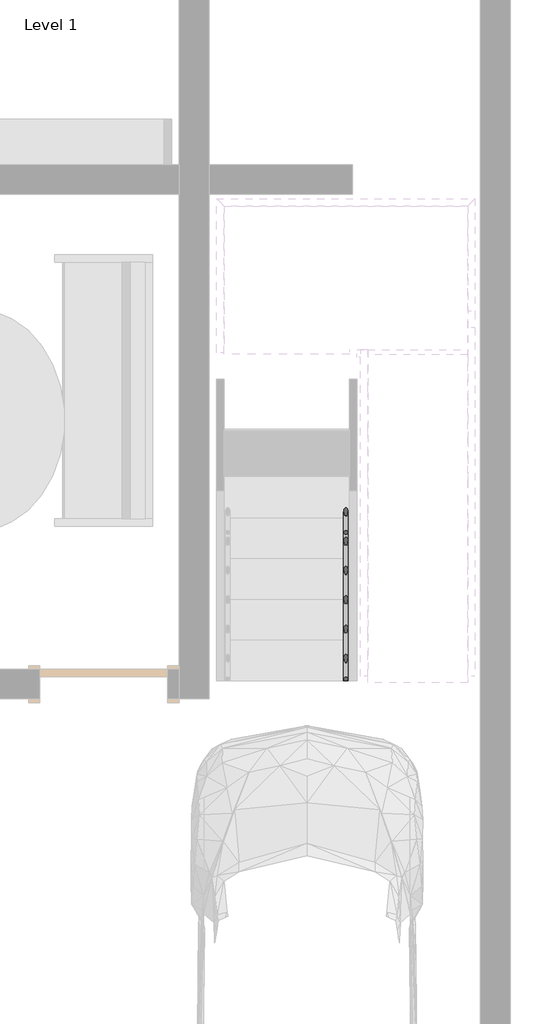
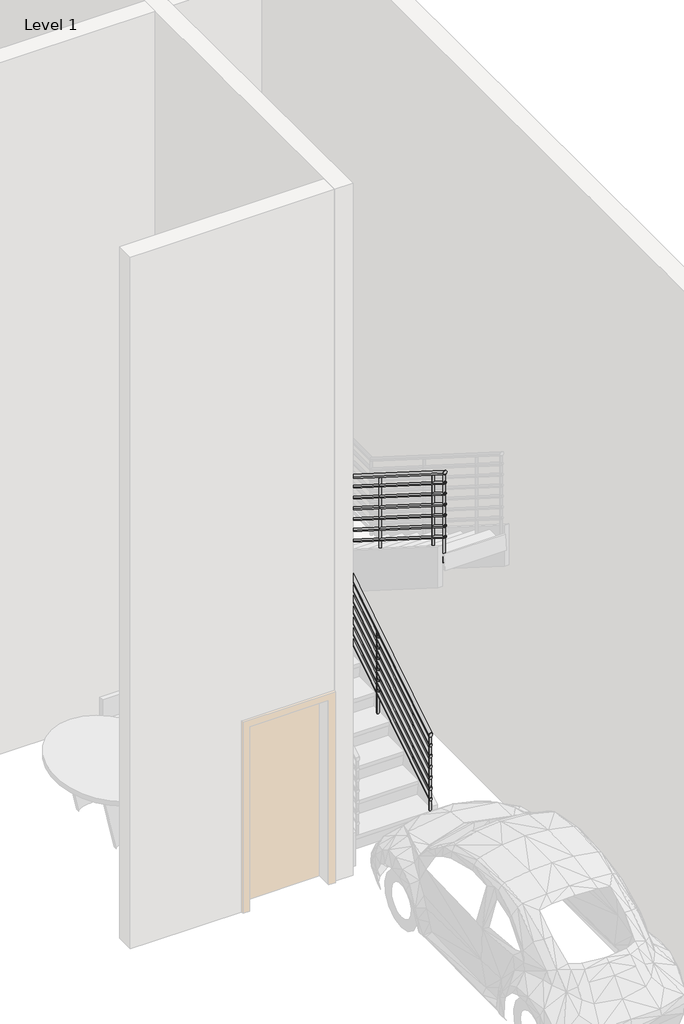
# One storey, part 2 of 4: 1 railing.
"""IFC4 building model written with IfcOpenShell, lengths in millimetres."""

from ifc_helpers import new_model, si_unit, point, frame, frame_2d, origin, place, context, project, spatial, circle_curve, ellipse_curve, trimmed, segment, composite_curve, outline, extrude, element, save
from ifc_brep_helpers import plane_surface, cylinder_surface, advanced_brep

model = new_model("IFC4")

# Units and contexts
model_context = context("Model", 3, world=origin())
ifc_project = project(units=[si_unit("LENGTHUNIT", "METRE", prefix="MILLI")], contexts=[model_context])

# Site, building, storey
site = spatial("IfcSite", under=ifc_project)
building = spatial("IfcBuilding", under=site)
storey = spatial("IfcBuildingStorey", under=building, Name="Level 1", Elevation=0.0)

# Railing
placement = place(None, origin())
element("IfcRailing", 1, ObjectType="900mm Pipe", at=placement, inside=storey, context=model_context, shape_type="SolidModel", body=[
    advanced_brep(
    [(474.1868738, 5121.4805518, 1224.1622432), (434.1868738, 5121.4805518, 1224.1622432), (474.1868738, 7327.2740048, 2619.1304348), (434.1868738, 7327.2740048, 2619.1304348), (474.1868738, 7356.6805518, 2619.1304348), (434.1868738, 7396.6805518, 2619.1304348), (627.5868738, 7356.6805518, 2619.1304348), (627.5868738, 7396.6805518, 2619.1304348)],
    [
        (0, 1, ellipse_curve(frame((454.1868738, 5121.4805518, 1224.1622432), z_axis=(0.0, -1.0, 0.0), x_axis=(0.0, 0.0, -1.0)), 23.6638438, 20.0)),
        (1, 0, ellipse_curve(frame((454.1868738, 5121.4805518, 1224.1622432), z_axis=(0.0, -1.0, 0.0), x_axis=(0.0, 0.0, -1.0)), 23.6638438, 20.0)),
        (0, 2),
        (2, 3, ellipse_curve(frame((454.1868738, 7327.2740048, 2619.1304348), z_axis=(0.0, -0.9605132043335073, -0.2782344053149755), x_axis=(0.0, 0.27823440531497556, -0.9605132043335073)), 20.822202, 20.0)),
        (3, 1),
        (3, 2, ellipse_curve(frame((454.1868738, 7327.2740048, 2619.1304348), z_axis=(0.0, -0.9605132043335073, -0.2782344053149755), x_axis=(0.0, 0.27823440531497556, -0.9605132043335073)), 20.822202, 20.0)),
        (2, 4),
        (4, 5, ellipse_curve(frame((454.1868738, 7376.6805518, 2619.1304348), z_axis=(-0.7071067811865482, -0.7071067811865467, 0.0), x_axis=(0.7071067811865466, -0.7071067811865485, 0.0)), 28.2842712, 20.0)),
        (5, 3),
        (5, 4, ellipse_curve(frame((454.1868738, 7376.6805518, 2619.1304348), z_axis=(-0.7071067811865482, -0.7071067811865467, 0.0), x_axis=(0.7071067811865466, -0.7071067811865485, 0.0)), 28.2842712, 20.0)),
        (6, 7, ellipse_curve(frame((627.5868738, 7376.6805518, 2619.1304348), z_axis=(0.7071067811865476, 0.0, 0.7071067811865476), x_axis=(-0.7071067811865474, 0.0, 0.7071067811865478)), 28.2842712, 20.0)),
        (7, 6, ellipse_curve(frame((627.5868738, 7376.6805518, 2619.1304348), z_axis=(0.7071067811865476, 0.0, 0.7071067811865476), x_axis=(-0.7071067811865474, 0.0, 0.7071067811865478)), 28.2842712, 20.0)),
        (4, 6),
        (7, 5),
    ],
    [
        plane_surface(frame((454.1868738, 5121.4805518, 1247.826087), z_axis=(0.0, -1.0, 0.0), x_axis=(0.0, 0.0, 1.0))),
        cylinder_surface(frame((454.1868738, 5132.1704646, 1230.9226623), z_axis=(0.0, -0.8451712313980438, -0.5344956404098301), x_axis=(-1.0, 0.0, 0.0)), 20.0),
        cylinder_surface(frame((454.1868738, 7321.4805518, 2619.1304348), z_axis=(0.0, -1.0, 0.0), x_axis=(-1.0, 0.0, 0.0)), 20.0),
        plane_surface(frame((607.5868738, 7376.6805518, 2639.1304348), z_axis=(0.7071067811865476, 0.0, 0.7071067811865476), x_axis=(0.7071067811865476, 0.0, -0.7071067811865476))),
        cylinder_surface(frame((454.1868738, 7376.6805518, 2619.1304348), z_axis=(-1.0, 0.0, 0.0), x_axis=(0.0, 1.0, 0.0)), 20.0),
    ],
    [
        (0, [[1, 2]]),
        (1, [[-1, 3, 4, 5]]),
        (1, [[-2, -5, 6, -3]]),
        (2, [[-4, 7, 8, 9]]),
        (2, [[-6, -9, 10, -7]]),
        (3, [[11, 12]]),
        (4, [[-8, 13, -12, 14]]),
        (4, [[-10, -14, -11, -13]]),
    ],
),
    advanced_brep(
    [(627.5868738, 7356.6805518, 2619.1304348), (627.5868738, 7396.6805518, 2619.1304348), (627.5868738, 7356.6805518, 2762.3007709), (627.5868738, 7396.6805518, 2784.3320158)],
    [
        (0, 1, ellipse_curve(frame((627.5868738, 7376.6805518, 2619.1304348), z_axis=(-0.7071067811865476, 0.0, -0.7071067811865476), x_axis=(0.7071067811865476, 0.0, -0.7071067811865474)), 28.2842712, 20.0)),
        (1, 0, ellipse_curve(frame((627.5868738, 7376.6805518, 2619.1304348), z_axis=(-0.7071067811865476, 0.0, -0.7071067811865476), x_axis=(0.7071067811865476, 0.0, -0.7071067811865474)), 28.2842712, 20.0)),
        (2, 3, ellipse_curve(frame((627.5868738, 7376.6805518, 2773.3163934), z_axis=(0.0, -0.4824439654458173, 0.8759268349610686), x_axis=(0.0, -0.8759268349610686, -0.48244396544581714)), 22.8329573, 20.0)),
        (3, 2, ellipse_curve(frame((627.5868738, 7376.6805518, 2773.3163934), z_axis=(0.0, -0.4824439654458173, 0.8759268349610686), x_axis=(0.0, -0.8759268349610686, -0.48244396544581714)), 22.8329573, 20.0)),
        (0, 2),
        (3, 1),
    ],
    [
        plane_surface(frame((627.5868738, 7376.6805518, 2619.1304348), z_axis=(-0.7071067811865476, 0.0, -0.7071067811865476), x_axis=(0.7071067811865476, 0.0, -0.7071067811865476))),
        plane_surface(frame((627.5868738, 7376.6805518, 2773.3163934), z_axis=(0.0, -0.4824439654458173, 0.8759268349610686), x_axis=(1.0, 0.0, 0.0))),
        cylinder_surface(frame((627.5868738, 7376.6805518, 2619.1304348), z_axis=(0.0, 0.0, -1.0), x_axis=(0.0, 1.0, 0.0)), 20.0),
    ],
    [
        (0, [[1, 2]]),
        (1, [[3, 4]]),
        (2, [[-1, 5, -4, 6]]),
        (2, [[-2, -6, -3, -5]]),
    ],
),
    advanced_brep(
    [(607.5868738, 7376.6805518, 2773.3163934), (647.5868738, 7376.6805518, 2773.3163934), (607.5868738, 5151.2805518, 4180.6839823), (647.5868738, 5151.2805518, 4180.6839823)],
    [
        (0, 1, ellipse_curve(frame((627.5868738, 7376.6805518, 2773.3163934), z_axis=(0.0, 0.4824439654458173, -0.8759268349610686), x_axis=(0.0, 0.8759268349610685, 0.4824439654458175)), 22.8329573, 20.0)),
        (1, 0, ellipse_curve(frame((627.5868738, 7376.6805518, 2773.3163934), z_axis=(0.0, 0.4824439654458173, -0.8759268349610686), x_axis=(0.0, 0.8759268349610685, 0.4824439654458175)), 22.8329573, 20.0)),
        (2, 3, ellipse_curve(frame((627.5868738, 5151.2805518, 4180.6839823), z_axis=(0.0, -1.0, 0.0), x_axis=(0.0, 0.0, -1.0)), 23.6638438, 20.0)),
        (3, 2, ellipse_curve(frame((627.5868738, 5151.2805518, 4180.6839823), z_axis=(0.0, -1.0, 0.0), x_axis=(0.0, 0.0, -1.0)), 23.6638438, 20.0)),
        (0, 2),
        (3, 1),
    ],
    [
        plane_surface(frame((627.5868738, 7396.6805518, 2784.3320158), z_axis=(0.0, 0.4824439654458173, -0.8759268349610686), x_axis=(1.0, 0.0, 0.0))),
        plane_surface(frame((627.5868738, 5151.2805518, 4204.3478261), z_axis=(0.0, -1.0, 0.0), x_axis=(0.0, 0.0, -1.0))),
        cylinder_surface(frame((627.5868738, 7385.990639, 2767.4285912), z_axis=(0.0, 0.8451712313980438, -0.5344956404098301), x_axis=(1.0, 0.0, 0.0)), 20.0),
    ],
    [
        (0, [[1, 2]]),
        (1, [[3, 4]]),
        (2, [[-1, 5, -4, 6]]),
        (2, [[-2, -6, -3, -5]]),
    ],
),
    advanced_brep(
    [(439.1868738, 5121.4805518, 1105.0782041), (469.1868738, 5121.4805518, 1105.0782041), (439.1868738, 7325.8256416, 2499.1304348), (469.1868738, 7325.8256416, 2499.1304348), (439.1868738, 7391.6805518, 2499.1304348), (469.1868738, 7361.6805518, 2499.1304348), (612.5868738, 7391.6805518, 2499.1304348), (612.5868738, 7361.6805518, 2499.1304348)],
    [
        (0, 1, ellipse_curve(frame((454.1868738, 5121.4805518, 1105.0782041), z_axis=(0.0, -1.0, 0.0), x_axis=(0.0, 0.0, -1.0)), 17.7478828, 15.0)),
        (1, 0, ellipse_curve(frame((454.1868738, 5121.4805518, 1105.0782041), z_axis=(0.0, -1.0, 0.0), x_axis=(0.0, 0.0, -1.0)), 17.7478828, 15.0)),
        (0, 2),
        (2, 3, ellipse_curve(frame((454.1868738, 7325.8256416, 2499.1304348), z_axis=(0.0, -0.9605132043335073, -0.2782344053149755), x_axis=(0.0, 0.27823440531497534, -0.9605132043335074)), 15.6166515, 15.0)),
        (3, 1),
        (3, 2, ellipse_curve(frame((454.1868738, 7325.8256416, 2499.1304348), z_axis=(0.0, -0.9605132043335073, -0.2782344053149755), x_axis=(0.0, 0.27823440531497534, -0.9605132043335074)), 15.6166515, 15.0)),
        (2, 4),
        (4, 5, ellipse_curve(frame((454.1868738, 7376.6805518, 2499.1304348), z_axis=(-0.7071067811865482, -0.7071067811865467, 0.0), x_axis=(0.7071067811865466, -0.7071067811865485, 0.0)), 21.2132034, 15.0)),
        (5, 3),
        (5, 4, ellipse_curve(frame((454.1868738, 7376.6805518, 2499.1304348), z_axis=(-0.7071067811865482, -0.7071067811865467, 0.0), x_axis=(0.7071067811865466, -0.7071067811865485, 0.0)), 21.2132034, 15.0)),
        (6, 7, circle_curve(frame((612.5868738, 7376.6805518, 2499.1304348), z_axis=(1.0, 0.0, 0.0), x_axis=(0.0, -1.0, 0.0)), 15.0)),
        (7, 6, circle_curve(frame((612.5868738, 7376.6805518, 2499.1304348), z_axis=(1.0, 0.0, 0.0), x_axis=(0.0, -1.0, 0.0)), 15.0)),
        (4, 6),
        (7, 5),
    ],
    [
        plane_surface(frame((454.1868738, 5121.4805518, 1122.826087), z_axis=(0.0, -1.0, 0.0), x_axis=(0.0, 0.0, 1.0))),
        cylinder_surface(frame((454.1868738, 5129.4979864, 1110.1485185), z_axis=(0.0, -0.845171231398044, -0.53449564040983), x_axis=(1.0, 0.0, 0.0)), 15.0),
        cylinder_surface(frame((454.1868738, 7321.4805518, 2499.1304348), z_axis=(0.0, -1.0, 0.0), x_axis=(1.0, 0.0, 0.0)), 15.0),
        plane_surface(frame((612.5868738, 7376.6805518, 2514.1304348), z_axis=(1.0, 0.0, 0.0), x_axis=(0.0, 1.0, 0.0))),
        cylinder_surface(frame((454.1868738, 7376.6805518, 2499.1304348), z_axis=(-1.0, 0.0, 0.0), x_axis=(0.0, -1.0, 0.0)), 15.0),
    ],
    [
        (0, [[1, 2]]),
        (1, [[-1, 3, 4, 5]]),
        (1, [[-2, -5, 6, -3]]),
        (2, [[-4, 7, 8, 9]]),
        (2, [[-6, -9, 10, -7]]),
        (3, [[11, 12]]),
        (4, [[-8, 13, -12, 14]]),
        (4, [[-10, -14, -11, -13]]),
    ],
),
    advanced_brep(
    [(642.5868738, 7391.6805518, 2644.7461883), (612.5868738, 7391.6805518, 2644.7461883), (642.5868738, 5151.2805518, 4061.5999432), (612.5868738, 5151.2805518, 4061.5999432)],
    [
        (0, 1, ellipse_curve(frame((627.5868738, 7391.6805518, 2644.7461883), z_axis=(0.0, 1.0, 0.0), x_axis=(0.0, 0.0, -1.0)), 17.7478828, 15.0)),
        (1, 0, ellipse_curve(frame((627.5868738, 7391.6805518, 2644.7461883), z_axis=(0.0, 1.0, 0.0), x_axis=(0.0, 0.0, -1.0)), 17.7478828, 15.0)),
        (2, 3, ellipse_curve(frame((627.5868738, 5151.2805518, 4061.5999432), z_axis=(0.0, -1.0, 0.0), x_axis=(0.0, 0.0, -1.0)), 17.7478828, 15.0)),
        (3, 2, ellipse_curve(frame((627.5868738, 5151.2805518, 4061.5999432), z_axis=(0.0, -1.0, 0.0), x_axis=(0.0, 0.0, -1.0)), 17.7478828, 15.0)),
        (0, 2),
        (3, 1),
    ],
    [
        plane_surface(frame((627.5868738, 7391.6805518, 2662.4940711), z_axis=(0.0, 1.0, 0.0), x_axis=(0.0, 0.0, -1.0))),
        plane_surface(frame((627.5868738, 5151.2805518, 4079.3478261), z_axis=(0.0, -1.0, 0.0), x_axis=(0.0, 0.0, -1.0))),
        cylinder_surface(frame((627.5868738, 7383.6631172, 2649.8165027), z_axis=(0.0, 0.8451712313980437, -0.5344956404098302), x_axis=(-1.0, 0.0, 0.0)), 15.0),
    ],
    [
        (0, [[1, 2]]),
        (1, [[3, 4]]),
        (2, [[-1, 5, -4, 6]]),
        (2, [[-2, -6, -3, -5]]),
    ],
),
    advanced_brep(
    [(439.1868738, 5121.4805518, 980.0782041), (469.1868738, 5121.4805518, 980.0782041), (439.1868738, 7325.8256416, 2374.1304348), (469.1868738, 7325.8256416, 2374.1304348), (439.1868738, 7391.6805518, 2374.1304348), (469.1868738, 7361.6805518, 2374.1304348), (612.5868738, 7391.6805518, 2374.1304348), (612.5868738, 7361.6805518, 2374.1304348)],
    [
        (0, 1, ellipse_curve(frame((454.1868738, 5121.4805518, 980.0782041), z_axis=(0.0, -1.0, 0.0), x_axis=(0.0, 0.0, -1.0)), 17.7478828, 15.0)),
        (1, 0, ellipse_curve(frame((454.1868738, 5121.4805518, 980.0782041), z_axis=(0.0, -1.0, 0.0), x_axis=(0.0, 0.0, -1.0)), 17.7478828, 15.0)),
        (0, 2),
        (2, 3, ellipse_curve(frame((454.1868738, 7325.8256416, 2374.1304348), z_axis=(0.0, -0.9605132043335073, -0.2782344053149755), x_axis=(0.0, 0.27823440531497556, -0.9605132043335073)), 15.6166515, 15.0)),
        (3, 1),
        (3, 2, ellipse_curve(frame((454.1868738, 7325.8256416, 2374.1304348), z_axis=(0.0, -0.9605132043335073, -0.2782344053149755), x_axis=(0.0, 0.27823440531497556, -0.9605132043335073)), 15.6166515, 15.0)),
        (2, 4),
        (4, 5, ellipse_curve(frame((454.1868738, 7376.6805518, 2374.1304348), z_axis=(-0.7071067811865482, -0.7071067811865467, 0.0), x_axis=(0.7071067811865466, -0.7071067811865485, 0.0)), 21.2132034, 15.0)),
        (5, 3),
        (5, 4, ellipse_curve(frame((454.1868738, 7376.6805518, 2374.1304348), z_axis=(-0.7071067811865482, -0.7071067811865467, 0.0), x_axis=(0.7071067811865466, -0.7071067811865485, 0.0)), 21.2132034, 15.0)),
        (6, 7, circle_curve(frame((612.5868738, 7376.6805518, 2374.1304348), z_axis=(1.0, 0.0, 0.0), x_axis=(0.0, -1.0, 0.0)), 15.0)),
        (7, 6, circle_curve(frame((612.5868738, 7376.6805518, 2374.1304348), z_axis=(1.0, 0.0, 0.0), x_axis=(0.0, -1.0, 0.0)), 15.0)),
        (4, 6),
        (7, 5),
    ],
    [
        plane_surface(frame((454.1868738, 5121.4805518, 997.826087), z_axis=(0.0, -1.0, 0.0), x_axis=(0.0, 0.0, 1.0))),
        cylinder_surface(frame((454.1868738, 5129.4979864, 985.1485185), z_axis=(0.0, -0.8451712313980438, -0.5344956404098301), x_axis=(1.0, 0.0, 0.0)), 15.0),
        cylinder_surface(frame((454.1868738, 7321.4805518, 2374.1304348), z_axis=(0.0, -1.0, 0.0), x_axis=(1.0, 0.0, 0.0)), 15.0),
        plane_surface(frame((612.5868738, 7376.6805518, 2389.1304348), z_axis=(1.0, 0.0, 0.0), x_axis=(0.0, 1.0, 0.0))),
        cylinder_surface(frame((454.1868738, 7376.6805518, 2374.1304348), z_axis=(-1.0, 0.0, 0.0), x_axis=(0.0, -1.0, 0.0)), 15.0),
    ],
    [
        (0, [[1, 2]]),
        (1, [[-1, 3, 4, 5]]),
        (1, [[-2, -5, 6, -3]]),
        (2, [[-4, 7, 8, 9]]),
        (2, [[-6, -9, 10, -7]]),
        (3, [[11, 12]]),
        (4, [[-8, 13, -12, 14]]),
        (4, [[-10, -14, -11, -13]]),
    ],
),
    advanced_brep(
    [(642.5868738, 7391.6805518, 2519.7461883), (612.5868738, 7391.6805518, 2519.7461883), (642.5868738, 5151.2805518, 3936.5999432), (612.5868738, 5151.2805518, 3936.5999432)],
    [
        (0, 1, ellipse_curve(frame((627.5868738, 7391.6805518, 2519.7461883), z_axis=(0.0, 1.0, 0.0), x_axis=(0.0, 0.0, -1.0)), 17.7478828, 15.0)),
        (1, 0, ellipse_curve(frame((627.5868738, 7391.6805518, 2519.7461883), z_axis=(0.0, 1.0, 0.0), x_axis=(0.0, 0.0, -1.0)), 17.7478828, 15.0)),
        (2, 3, ellipse_curve(frame((627.5868738, 5151.2805518, 3936.5999432), z_axis=(0.0, -1.0, 0.0), x_axis=(0.0, 0.0, -1.0)), 17.7478828, 15.0)),
        (3, 2, ellipse_curve(frame((627.5868738, 5151.2805518, 3936.5999432), z_axis=(0.0, -1.0, 0.0), x_axis=(0.0, 0.0, -1.0)), 17.7478828, 15.0)),
        (0, 2),
        (3, 1),
    ],
    [
        plane_surface(frame((627.5868738, 7391.6805518, 2537.4940711), z_axis=(0.0, 1.0, 0.0), x_axis=(0.0, 0.0, -1.0))),
        plane_surface(frame((627.5868738, 5151.2805518, 3954.3478261), z_axis=(0.0, -1.0, 0.0), x_axis=(0.0, 0.0, -1.0))),
        cylinder_surface(frame((627.5868738, 7383.6631172, 2524.8165027), z_axis=(0.0, 0.8451712313980438, -0.5344956404098301), x_axis=(-1.0, 0.0, 0.0)), 15.0),
    ],
    [
        (0, [[1, 2]]),
        (1, [[3, 4]]),
        (2, [[-1, 5, -4, 6]]),
        (2, [[-2, -6, -3, -5]]),
    ],
),
    advanced_brep(
    [(439.1868738, 5121.4805518, 855.0782041), (469.1868738, 5121.4805518, 855.0782041), (439.1868738, 7325.8256416, 2249.1304348), (469.1868738, 7325.8256416, 2249.1304348), (439.1868738, 7391.6805518, 2249.1304348), (469.1868738, 7361.6805518, 2249.1304348), (612.5868738, 7391.6805518, 2249.1304348), (612.5868738, 7361.6805518, 2249.1304348)],
    [
        (0, 1, ellipse_curve(frame((454.1868738, 5121.4805518, 855.0782041), z_axis=(0.0, -1.0, 0.0), x_axis=(0.0, 0.0, -1.0)), 17.7478828, 15.0)),
        (1, 0, ellipse_curve(frame((454.1868738, 5121.4805518, 855.0782041), z_axis=(0.0, -1.0, 0.0), x_axis=(0.0, 0.0, -1.0)), 17.7478828, 15.0)),
        (0, 2),
        (2, 3, ellipse_curve(frame((454.1868738, 7325.8256416, 2249.1304348), z_axis=(0.0, -0.9605132043335073, -0.2782344053149755), x_axis=(0.0, 0.27823440531497556, -0.9605132043335073)), 15.6166515, 15.0)),
        (3, 1),
        (3, 2, ellipse_curve(frame((454.1868738, 7325.8256416, 2249.1304348), z_axis=(0.0, -0.9605132043335073, -0.2782344053149755), x_axis=(0.0, 0.27823440531497556, -0.9605132043335073)), 15.6166515, 15.0)),
        (2, 4),
        (4, 5, ellipse_curve(frame((454.1868738, 7376.6805518, 2249.1304348), z_axis=(-0.7071067811865482, -0.7071067811865467, 0.0), x_axis=(0.7071067811865466, -0.7071067811865485, 0.0)), 21.2132034, 15.0)),
        (5, 3),
        (5, 4, ellipse_curve(frame((454.1868738, 7376.6805518, 2249.1304348), z_axis=(-0.7071067811865482, -0.7071067811865467, 0.0), x_axis=(0.7071067811865466, -0.7071067811865485, 0.0)), 21.2132034, 15.0)),
        (6, 7, circle_curve(frame((612.5868738, 7376.6805518, 2249.1304348), z_axis=(1.0, 0.0, 0.0), x_axis=(0.0, -1.0, 0.0)), 15.0)),
        (7, 6, circle_curve(frame((612.5868738, 7376.6805518, 2249.1304348), z_axis=(1.0, 0.0, 0.0), x_axis=(0.0, -1.0, 0.0)), 15.0)),
        (4, 6),
        (7, 5),
    ],
    [
        plane_surface(frame((454.1868738, 5121.4805518, 872.826087), z_axis=(0.0, -1.0, 0.0), x_axis=(0.0, 0.0, 1.0))),
        cylinder_surface(frame((454.1868738, 5129.4979864, 860.1485185), z_axis=(0.0, -0.8451712313980438, -0.5344956404098301), x_axis=(1.0, 0.0, 0.0)), 15.0),
        cylinder_surface(frame((454.1868738, 7321.4805518, 2249.1304348), z_axis=(0.0, -1.0, 0.0), x_axis=(1.0, 0.0, 0.0)), 15.0),
        plane_surface(frame((612.5868738, 7376.6805518, 2264.1304348), z_axis=(1.0, 0.0, 0.0), x_axis=(0.0, 1.0, 0.0))),
        cylinder_surface(frame((454.1868738, 7376.6805518, 2249.1304348), z_axis=(-1.0, 0.0, 0.0), x_axis=(0.0, -1.0, 0.0)), 15.0),
    ],
    [
        (0, [[1, 2]]),
        (1, [[-1, 3, 4, 5]]),
        (1, [[-2, -5, 6, -3]]),
        (2, [[-4, 7, 8, 9]]),
        (2, [[-6, -9, 10, -7]]),
        (3, [[11, 12]]),
        (4, [[-8, 13, -12, 14]]),
        (4, [[-10, -14, -11, -13]]),
    ],
),
    advanced_brep(
    [(642.5868738, 7391.6805518, 2394.7461883), (612.5868738, 7391.6805518, 2394.7461883), (642.5868738, 5151.2805518, 3811.5999432), (612.5868738, 5151.2805518, 3811.5999432)],
    [
        (0, 1, ellipse_curve(frame((627.5868738, 7391.6805518, 2394.7461883), z_axis=(0.0, 1.0, 0.0), x_axis=(0.0, 0.0, -1.0)), 17.7478828, 15.0)),
        (1, 0, ellipse_curve(frame((627.5868738, 7391.6805518, 2394.7461883), z_axis=(0.0, 1.0, 0.0), x_axis=(0.0, 0.0, -1.0)), 17.7478828, 15.0)),
        (2, 3, ellipse_curve(frame((627.5868738, 5151.2805518, 3811.5999432), z_axis=(0.0, -1.0, 0.0), x_axis=(0.0, 0.0, -1.0)), 17.7478828, 15.0)),
        (3, 2, ellipse_curve(frame((627.5868738, 5151.2805518, 3811.5999432), z_axis=(0.0, -1.0, 0.0), x_axis=(0.0, 0.0, -1.0)), 17.7478828, 15.0)),
        (0, 2),
        (3, 1),
    ],
    [
        plane_surface(frame((627.5868738, 7391.6805518, 2412.4940711), z_axis=(0.0, 1.0, 0.0), x_axis=(0.0, 0.0, -1.0))),
        plane_surface(frame((627.5868738, 5151.2805518, 3829.3478261), z_axis=(0.0, -1.0, 0.0), x_axis=(0.0, 0.0, -1.0))),
        cylinder_surface(frame((627.5868738, 7383.6631172, 2399.8165027), z_axis=(0.0, 0.8451712313980438, -0.53449564040983), x_axis=(-1.0, 0.0, 0.0)), 15.0),
    ],
    [
        (0, [[1, 2]]),
        (1, [[3, 4]]),
        (2, [[-1, 5, -4, 6]]),
        (2, [[-2, -6, -3, -5]]),
    ],
),
    advanced_brep(
    [(439.1868738, 5121.4805518, 730.0782041), (469.1868738, 5121.4805518, 730.0782041), (439.1868738, 7325.8256416, 2124.1304348), (469.1868738, 7325.8256416, 2124.1304348), (439.1868738, 7391.6805518, 2124.1304348), (469.1868738, 7361.6805518, 2124.1304348), (612.5868738, 7391.6805518, 2124.1304348), (612.5868738, 7361.6805518, 2124.1304348)],
    [
        (0, 1, ellipse_curve(frame((454.1868738, 5121.4805518, 730.0782041), z_axis=(0.0, -1.0, 0.0), x_axis=(0.0, 0.0, -1.0)), 17.7478828, 15.0)),
        (1, 0, ellipse_curve(frame((454.1868738, 5121.4805518, 730.0782041), z_axis=(0.0, -1.0, 0.0), x_axis=(0.0, 0.0, -1.0)), 17.7478828, 15.0)),
        (0, 2),
        (2, 3, ellipse_curve(frame((454.1868738, 7325.8256416, 2124.1304348), z_axis=(0.0, -0.9605132043335073, -0.2782344053149755), x_axis=(0.0, 0.27823440531497556, -0.9605132043335073)), 15.6166515, 15.0)),
        (3, 1),
        (3, 2, ellipse_curve(frame((454.1868738, 7325.8256416, 2124.1304348), z_axis=(0.0, -0.9605132043335073, -0.2782344053149755), x_axis=(0.0, 0.27823440531497556, -0.9605132043335073)), 15.6166515, 15.0)),
        (2, 4),
        (4, 5, ellipse_curve(frame((454.1868738, 7376.6805518, 2124.1304348), z_axis=(-0.7071067811865482, -0.7071067811865467, 0.0), x_axis=(0.7071067811865466, -0.7071067811865485, 0.0)), 21.2132034, 15.0)),
        (5, 3),
        (5, 4, ellipse_curve(frame((454.1868738, 7376.6805518, 2124.1304348), z_axis=(-0.7071067811865482, -0.7071067811865467, 0.0), x_axis=(0.7071067811865466, -0.7071067811865485, 0.0)), 21.2132034, 15.0)),
        (6, 7, circle_curve(frame((612.5868738, 7376.6805518, 2124.1304348), z_axis=(1.0, 0.0, 0.0), x_axis=(0.0, -1.0, 0.0)), 15.0)),
        (7, 6, circle_curve(frame((612.5868738, 7376.6805518, 2124.1304348), z_axis=(1.0, 0.0, 0.0), x_axis=(0.0, -1.0, 0.0)), 15.0)),
        (4, 6),
        (7, 5),
    ],
    [
        plane_surface(frame((454.1868738, 5121.4805518, 747.826087), z_axis=(0.0, -1.0, 0.0), x_axis=(0.0, 0.0, 1.0))),
        cylinder_surface(frame((454.1868738, 5129.4979864, 735.1485185), z_axis=(0.0, -0.8451712313980438, -0.5344956404098301), x_axis=(1.0, 0.0, 0.0)), 15.0),
        cylinder_surface(frame((454.1868738, 7321.4805518, 2124.1304348), z_axis=(0.0, -1.0, 0.0), x_axis=(1.0, 0.0, 0.0)), 15.0),
        plane_surface(frame((612.5868738, 7376.6805518, 2139.1304348), z_axis=(1.0, 0.0, 0.0), x_axis=(0.0, 1.0, 0.0))),
        cylinder_surface(frame((454.1868738, 7376.6805518, 2124.1304348), z_axis=(-1.0, 0.0, 0.0), x_axis=(0.0, -1.0, 0.0)), 15.0),
    ],
    [
        (0, [[1, 2]]),
        (1, [[-1, 3, 4, 5]]),
        (1, [[-2, -5, 6, -3]]),
        (2, [[-4, 7, 8, 9]]),
        (2, [[-6, -9, 10, -7]]),
        (3, [[11, 12]]),
        (4, [[-8, 13, -12, 14]]),
        (4, [[-10, -14, -11, -13]]),
    ],
),
    advanced_brep(
    [(642.5868738, 7391.6805518, 2269.7461883), (612.5868738, 7391.6805518, 2269.7461883), (642.5868738, 5151.2805518, 3686.5999432), (612.5868738, 5151.2805518, 3686.5999432)],
    [
        (0, 1, ellipse_curve(frame((627.5868738, 7391.6805518, 2269.7461883), z_axis=(0.0, 1.0, 0.0), x_axis=(0.0, 0.0, -1.0)), 17.7478828, 15.0)),
        (1, 0, ellipse_curve(frame((627.5868738, 7391.6805518, 2269.7461883), z_axis=(0.0, 1.0, 0.0), x_axis=(0.0, 0.0, -1.0)), 17.7478828, 15.0)),
        (2, 3, ellipse_curve(frame((627.5868738, 5151.2805518, 3686.5999432), z_axis=(0.0, -1.0, 0.0), x_axis=(0.0, 0.0, -1.0)), 17.7478828, 15.0)),
        (3, 2, ellipse_curve(frame((627.5868738, 5151.2805518, 3686.5999432), z_axis=(0.0, -1.0, 0.0), x_axis=(0.0, 0.0, -1.0)), 17.7478828, 15.0)),
        (0, 2),
        (3, 1),
    ],
    [
        plane_surface(frame((627.5868738, 7391.6805518, 2287.4940711), z_axis=(0.0, 1.0, 0.0), x_axis=(0.0, 0.0, -1.0))),
        plane_surface(frame((627.5868738, 5151.2805518, 3704.3478261), z_axis=(0.0, -1.0, 0.0), x_axis=(0.0, 0.0, -1.0))),
        cylinder_surface(frame((627.5868738, 7383.6631172, 2274.8165027), z_axis=(0.0, 0.8451712313980438, -0.5344956404098301), x_axis=(-1.0, 0.0, 0.0)), 15.0),
    ],
    [
        (0, [[1, 2]]),
        (1, [[3, 4]]),
        (2, [[-1, 5, -4, 6]]),
        (2, [[-2, -6, -3, -5]]),
    ],
),
    advanced_brep(
    [(439.1868738, 5121.4805518, 605.0782041), (469.1868738, 5121.4805518, 605.0782041), (439.1868738, 7325.8256416, 1999.1304348), (469.1868738, 7325.8256416, 1999.1304348), (439.1868738, 7391.6805518, 1999.1304348), (469.1868738, 7361.6805518, 1999.1304348), (612.5868738, 7391.6805518, 1999.1304348), (612.5868738, 7361.6805518, 1999.1304348)],
    [
        (0, 1, ellipse_curve(frame((454.1868738, 5121.4805518, 605.0782041), z_axis=(0.0, -1.0, 0.0), x_axis=(0.0, 0.0, -1.0)), 17.7478828, 15.0)),
        (1, 0, ellipse_curve(frame((454.1868738, 5121.4805518, 605.0782041), z_axis=(0.0, -1.0, 0.0), x_axis=(0.0, 0.0, -1.0)), 17.7478828, 15.0)),
        (0, 2),
        (2, 3, ellipse_curve(frame((454.1868738, 7325.8256416, 1999.1304348), z_axis=(0.0, -0.9605132043335073, -0.2782344053149755), x_axis=(0.0, 0.27823440531497556, -0.9605132043335073)), 15.6166515, 15.0)),
        (3, 1),
        (3, 2, ellipse_curve(frame((454.1868738, 7325.8256416, 1999.1304348), z_axis=(0.0, -0.9605132043335073, -0.2782344053149755), x_axis=(0.0, 0.27823440531497556, -0.9605132043335073)), 15.6166515, 15.0)),
        (2, 4),
        (4, 5, ellipse_curve(frame((454.1868738, 7376.6805518, 1999.1304348), z_axis=(-0.7071067811865482, -0.7071067811865467, 0.0), x_axis=(0.7071067811865466, -0.7071067811865485, 0.0)), 21.2132034, 15.0)),
        (5, 3),
        (5, 4, ellipse_curve(frame((454.1868738, 7376.6805518, 1999.1304348), z_axis=(-0.7071067811865482, -0.7071067811865467, 0.0), x_axis=(0.7071067811865466, -0.7071067811865485, 0.0)), 21.2132034, 15.0)),
        (6, 7, circle_curve(frame((612.5868738, 7376.6805518, 1999.1304348), z_axis=(1.0, 0.0, 0.0), x_axis=(0.0, -1.0, 0.0)), 15.0)),
        (7, 6, circle_curve(frame((612.5868738, 7376.6805518, 1999.1304348), z_axis=(1.0, 0.0, 0.0), x_axis=(0.0, -1.0, 0.0)), 15.0)),
        (4, 6),
        (7, 5),
    ],
    [
        plane_surface(frame((454.1868738, 5121.4805518, 622.826087), z_axis=(0.0, -1.0, 0.0), x_axis=(0.0, 0.0, 1.0))),
        cylinder_surface(frame((454.1868738, 5129.4979864, 610.1485185), z_axis=(0.0, -0.8451712313980438, -0.5344956404098301), x_axis=(1.0, 0.0, 0.0)), 15.0),
        cylinder_surface(frame((454.1868738, 7321.4805518, 1999.1304348), z_axis=(0.0, -1.0, 0.0), x_axis=(1.0, 0.0, 0.0)), 15.0),
        plane_surface(frame((612.5868738, 7376.6805518, 2014.1304348), z_axis=(1.0, 0.0, 0.0), x_axis=(0.0, 1.0, 0.0))),
        cylinder_surface(frame((454.1868738, 7376.6805518, 1999.1304348), z_axis=(-1.0, 0.0, 0.0), x_axis=(0.0, -1.0, 0.0)), 15.0),
    ],
    [
        (0, [[1, 2]]),
        (1, [[-1, 3, 4, 5]]),
        (1, [[-2, -5, 6, -3]]),
        (2, [[-4, 7, 8, 9]]),
        (2, [[-6, -9, 10, -7]]),
        (3, [[11, 12]]),
        (4, [[-8, 13, -12, 14]]),
        (4, [[-10, -14, -11, -13]]),
    ],
),
    advanced_brep(
    [(642.5868738, 7391.6805518, 2144.7461883), (612.5868738, 7391.6805518, 2144.7461883), (642.5868738, 5151.2805518, 3561.5999432), (612.5868738, 5151.2805518, 3561.5999432)],
    [
        (0, 1, ellipse_curve(frame((627.5868738, 7391.6805518, 2144.7461883), z_axis=(0.0, 1.0, 0.0), x_axis=(0.0, 0.0, -1.0)), 17.7478828, 15.0)),
        (1, 0, ellipse_curve(frame((627.5868738, 7391.6805518, 2144.7461883), z_axis=(0.0, 1.0, 0.0), x_axis=(0.0, 0.0, -1.0)), 17.7478828, 15.0)),
        (2, 3, ellipse_curve(frame((627.5868738, 5151.2805518, 3561.5999432), z_axis=(0.0, -1.0, 0.0), x_axis=(0.0, 0.0, -1.0)), 17.7478828, 15.0)),
        (3, 2, ellipse_curve(frame((627.5868738, 5151.2805518, 3561.5999432), z_axis=(0.0, -1.0, 0.0), x_axis=(0.0, 0.0, -1.0)), 17.7478828, 15.0)),
        (0, 2),
        (3, 1),
    ],
    [
        plane_surface(frame((627.5868738, 7391.6805518, 2162.4940711), z_axis=(0.0, 1.0, 0.0), x_axis=(0.0, 0.0, -1.0))),
        plane_surface(frame((627.5868738, 5151.2805518, 3579.3478261), z_axis=(0.0, -1.0, 0.0), x_axis=(0.0, 0.0, -1.0))),
        cylinder_surface(frame((627.5868738, 7383.6631172, 2149.8165027), z_axis=(0.0, 0.8451712313980437, -0.5344956404098301), x_axis=(-1.0, 0.0, 0.0)), 15.0),
    ],
    [
        (0, [[1, 2]]),
        (1, [[3, 4]]),
        (2, [[-1, 5, -4, 6]]),
        (2, [[-2, -6, -3, -5]]),
    ],
),
    advanced_brep(
    [(439.1868738, 5121.4805518, 480.0782041), (469.1868738, 5121.4805518, 480.0782041), (439.1868738, 7325.8256416, 1874.1304348), (469.1868738, 7325.8256416, 1874.1304348), (439.1868738, 7391.6805518, 1874.1304348), (469.1868738, 7361.6805518, 1874.1304348), (612.5868738, 7391.6805518, 1874.1304348), (612.5868738, 7361.6805518, 1874.1304348)],
    [
        (0, 1, ellipse_curve(frame((454.1868738, 5121.4805518, 480.0782041), z_axis=(0.0, -1.0, 0.0), x_axis=(0.0, 0.0, -1.0)), 17.7478828, 15.0)),
        (1, 0, ellipse_curve(frame((454.1868738, 5121.4805518, 480.0782041), z_axis=(0.0, -1.0, 0.0), x_axis=(0.0, 0.0, -1.0)), 17.7478828, 15.0)),
        (0, 2),
        (2, 3, ellipse_curve(frame((454.1868738, 7325.8256416, 1874.1304348), z_axis=(0.0, -0.9605132043335073, -0.2782344053149755), x_axis=(0.0, 0.27823440531497556, -0.9605132043335073)), 15.6166515, 15.0)),
        (3, 1),
        (3, 2, ellipse_curve(frame((454.1868738, 7325.8256416, 1874.1304348), z_axis=(0.0, -0.9605132043335073, -0.2782344053149755), x_axis=(0.0, 0.27823440531497556, -0.9605132043335073)), 15.6166515, 15.0)),
        (2, 4),
        (4, 5, ellipse_curve(frame((454.1868738, 7376.6805518, 1874.1304348), z_axis=(-0.7071067811865482, -0.7071067811865467, 0.0), x_axis=(0.7071067811865466, -0.7071067811865485, 0.0)), 21.2132034, 15.0)),
        (5, 3),
        (5, 4, ellipse_curve(frame((454.1868738, 7376.6805518, 1874.1304348), z_axis=(-0.7071067811865482, -0.7071067811865467, 0.0), x_axis=(0.7071067811865466, -0.7071067811865485, 0.0)), 21.2132034, 15.0)),
        (6, 7, circle_curve(frame((612.5868738, 7376.6805518, 1874.1304348), z_axis=(1.0, 0.0, 0.0), x_axis=(0.0, -1.0, 0.0)), 15.0)),
        (7, 6, circle_curve(frame((612.5868738, 7376.6805518, 1874.1304348), z_axis=(1.0, 0.0, 0.0), x_axis=(0.0, -1.0, 0.0)), 15.0)),
        (4, 6),
        (7, 5),
    ],
    [
        plane_surface(frame((454.1868738, 5121.4805518, 497.826087), z_axis=(0.0, -1.0, 0.0), x_axis=(0.0, 0.0, 1.0))),
        cylinder_surface(frame((454.1868738, 5129.4979864, 485.1485185), z_axis=(0.0, -0.8451712313980438, -0.5344956404098301), x_axis=(1.0, 0.0, 0.0)), 15.0),
        cylinder_surface(frame((454.1868738, 7321.4805518, 1874.1304348), z_axis=(0.0, -1.0, 0.0), x_axis=(1.0, 0.0, 0.0)), 15.0),
        plane_surface(frame((612.5868738, 7376.6805518, 1889.1304348), z_axis=(1.0, 0.0, 0.0), x_axis=(0.0, 1.0, 0.0))),
        cylinder_surface(frame((454.1868738, 7376.6805518, 1874.1304348), z_axis=(-1.0, 0.0, 0.0), x_axis=(0.0, -1.0, 0.0)), 15.0),
    ],
    [
        (0, [[1, 2]]),
        (1, [[-1, 3, 4, 5]]),
        (1, [[-2, -5, 6, -3]]),
        (2, [[-4, 7, 8, 9]]),
        (2, [[-6, -9, 10, -7]]),
        (3, [[11, 12]]),
        (4, [[-8, 13, -12, 14]]),
        (4, [[-10, -14, -11, -13]]),
    ],
),
    advanced_brep(
    [(642.5868738, 7391.6805518, 2019.7461883), (612.5868738, 7391.6805518, 2019.7461883), (642.5868738, 5151.2805518, 3436.5999432), (612.5868738, 5151.2805518, 3436.5999432)],
    [
        (0, 1, ellipse_curve(frame((627.5868738, 7391.6805518, 2019.7461883), z_axis=(0.0, 1.0, 0.0), x_axis=(0.0, 0.0, -1.0)), 17.7478828, 15.0)),
        (1, 0, ellipse_curve(frame((627.5868738, 7391.6805518, 2019.7461883), z_axis=(0.0, 1.0, 0.0), x_axis=(0.0, 0.0, -1.0)), 17.7478828, 15.0)),
        (2, 3, ellipse_curve(frame((627.5868738, 5151.2805518, 3436.5999432), z_axis=(0.0, -1.0, 0.0), x_axis=(0.0, 0.0, -1.0)), 17.7478828, 15.0)),
        (3, 2, ellipse_curve(frame((627.5868738, 5151.2805518, 3436.5999432), z_axis=(0.0, -1.0, 0.0), x_axis=(0.0, 0.0, -1.0)), 17.7478828, 15.0)),
        (0, 2),
        (3, 1),
    ],
    [
        plane_surface(frame((627.5868738, 7391.6805518, 2037.4940711), z_axis=(0.0, 1.0, 0.0), x_axis=(0.0, 0.0, -1.0))),
        plane_surface(frame((627.5868738, 5151.2805518, 3454.3478261), z_axis=(0.0, -1.0, 0.0), x_axis=(0.0, 0.0, -1.0))),
        cylinder_surface(frame((627.5868738, 7383.6631172, 2024.8165027), z_axis=(0.0, 0.8451712313980438, -0.5344956404098301), x_axis=(-1.0, 0.0, 0.0)), 15.0),
    ],
    [
        (0, [[1, 2]]),
        (1, [[3, 4]]),
        (2, [[-1, 5, -4, 6]]),
        (2, [[-2, -6, -3, -5]]),
    ],
),
    advanced_brep(
    [(615.0868738, 5376.6805518, 4014.474684), (615.0868738, 5376.6805518, 3130.4347826), (640.0868738, 5376.6805518, 3130.4347826), (640.0868738, 5376.6805518, 4014.474684)],
    [
        (0, 1),
        (1, 2, circle_curve(frame((627.5868738, 5376.6805518, 3130.4347826), z_axis=(0.0, 0.0, 1.0), x_axis=(1.0, 0.0, 0.0)), 12.5)),
        (2, 3),
        (3, 0, ellipse_curve(frame((627.5868738, 5376.6805518, 4014.474684), z_axis=(0.0, -0.5344956404098302, -0.8451712313980437), x_axis=(0.0, -0.8451712313980437, 0.53449564040983)), 14.7899024, 12.5)),
        (0, 3, ellipse_curve(frame((627.5868738, 5376.6805518, 4014.474684), z_axis=(0.0, -0.5344956404098302, -0.8451712313980437), x_axis=(0.0, -0.8451712313980437, 0.53449564040983)), 14.7899024, 12.5)),
        (2, 1, circle_curve(frame((627.5868738, 5376.6805518, 3130.4347826), z_axis=(0.0, 0.0, 1.0), x_axis=(1.0, 0.0, 0.0)), 12.5)),
    ],
    [
        cylinder_surface(frame((627.5868738, 5376.6805518, 3030.4347826), z_axis=(0.0, 0.0, 1.0), x_axis=(1.0, 0.0, 0.0)), 12.5),
        plane_surface(frame((652.5868738, 5351.6805518, 4030.2849606), z_axis=(0.0, 0.5344956404098302, 0.8451712313980437), x_axis=(-1.0, 0.0, 0.0))),
        plane_surface(frame((652.5868738, 5401.6805518, 3130.4347826), z_axis=(0.0, 0.0, -1.0), x_axis=(-1.0, 0.0, 0.0))),
    ],
    [
        (0, [[1, 2, 3, 4]]),
        (0, [[-1, 5, -3, 6]]),
        (1, [[-4, -5]]),
        (2, [[-2, -6]]),
    ],
),
    advanced_brep(
    [(615.0868738, 6376.6805518, 3382.0636168), (615.0868738, 6376.6805518, 2434.7826087), (640.0868738, 6376.6805518, 2434.7826087), (640.0868738, 6376.6805518, 3382.0636168)],
    [
        (0, 1),
        (1, 2, circle_curve(frame((627.5868738, 6376.6805518, 2434.7826087), z_axis=(0.0, 0.0, 1.0), x_axis=(1.0, 0.0, 0.0)), 12.5)),
        (2, 3),
        (3, 0, ellipse_curve(frame((627.5868738, 6376.6805518, 3382.0636168), z_axis=(0.0, -0.5344956404098302, -0.8451712313980437), x_axis=(0.0, -0.8451712313980437, 0.53449564040983)), 14.7899024, 12.5)),
        (0, 3, ellipse_curve(frame((627.5868738, 6376.6805518, 3382.0636168), z_axis=(0.0, -0.5344956404098302, -0.8451712313980437), x_axis=(0.0, -0.8451712313980437, 0.53449564040983)), 14.7899024, 12.5)),
        (2, 1, circle_curve(frame((627.5868738, 6376.6805518, 2434.7826087), z_axis=(0.0, 0.0, 1.0), x_axis=(1.0, 0.0, 0.0)), 12.5)),
    ],
    [
        cylinder_surface(frame((627.5868738, 6376.6805518, 2334.7826087), z_axis=(0.0, 0.0, 1.0), x_axis=(1.0, 0.0, 0.0)), 12.5),
        plane_surface(frame((652.5868738, 6351.6805518, 3397.8738934), z_axis=(0.0, 0.5344956404098302, 0.8451712313980437), x_axis=(-1.0, 0.0, 0.0))),
        plane_surface(frame((652.5868738, 6401.6805518, 2434.7826087), z_axis=(0.0, 0.0, -1.0), x_axis=(-1.0, 0.0, 0.0))),
    ],
    [
        (0, [[1, 2, 3, 4]]),
        (0, [[-1, 5, -3, 6]]),
        (1, [[-4, -5]]),
        (2, [[-2, -6]]),
    ],
),
    advanced_brep(
    [(466.6868738, 7121.4805518, 2465.3205338), (466.6868738, 7121.4805518, 1565.2173913), (441.6868738, 7121.4805518, 1565.2173913), (441.6868738, 7121.4805518, 2465.3205338)],
    [
        (0, 1),
        (1, 2, circle_curve(frame((454.1868738, 7121.4805518, 1565.2173913), z_axis=(0.0, 0.0, 1.0), x_axis=(-1.0, 0.0, 0.0)), 12.5)),
        (2, 3),
        (3, 0, ellipse_curve(frame((454.1868738, 7121.4805518, 2465.3205338), z_axis=(0.0, 0.5344956404098302, -0.8451712313980437), x_axis=(0.0, 0.8451712313980437, 0.53449564040983)), 14.7899024, 12.5)),
        (0, 3, ellipse_curve(frame((454.1868738, 7121.4805518, 2465.3205338), z_axis=(0.0, 0.5344956404098302, -0.8451712313980437), x_axis=(0.0, 0.8451712313980437, 0.53449564040983)), 14.7899024, 12.5)),
        (2, 1, circle_curve(frame((454.1868738, 7121.4805518, 1565.2173913), z_axis=(0.0, 0.0, 1.0), x_axis=(-1.0, 0.0, 0.0)), 12.5)),
    ],
    [
        cylinder_surface(frame((454.1868738, 7121.4805518, 1465.2173913), z_axis=(0.0, 0.0, 1.0), x_axis=(-1.0, 0.0, 0.0)), 12.5),
        plane_surface(frame((429.1868738, 7146.4805518, 2481.1308104), z_axis=(0.0, -0.5344956404098302, 0.8451712313980437), x_axis=(1.0, 0.0, 0.0))),
        plane_surface(frame((429.1868738, 7096.4805518, 1565.2173913), z_axis=(0.0, 0.0, -1.0), x_axis=(1.0, 0.0, 0.0))),
    ],
    [
        (0, [[1, 2, 3, 4]]),
        (0, [[-1, 5, -3, 6]]),
        (1, [[-4, -5]]),
        (2, [[-2, -6]]),
    ],
),
    advanced_brep(
    [(466.6868738, 6121.4805518, 1832.9094666), (466.6868738, 6121.4805518, 869.5652174), (441.6868738, 6121.4805518, 869.5652174), (441.6868738, 6121.4805518, 1832.9094666)],
    [
        (0, 1),
        (1, 2, circle_curve(frame((454.1868738, 6121.4805518, 869.5652174), z_axis=(0.0, 0.0, 1.0), x_axis=(-1.0, 0.0, 0.0)), 12.5)),
        (2, 3),
        (3, 0, ellipse_curve(frame((454.1868738, 6121.4805518, 1832.9094666), z_axis=(0.0, 0.5344956404098302, -0.8451712313980437), x_axis=(0.0, 0.8451712313980437, 0.53449564040983)), 14.7899024, 12.5)),
        (0, 3, ellipse_curve(frame((454.1868738, 6121.4805518, 1832.9094666), z_axis=(0.0, 0.5344956404098302, -0.8451712313980437), x_axis=(0.0, 0.8451712313980437, 0.53449564040983)), 14.7899024, 12.5)),
        (2, 1, circle_curve(frame((454.1868738, 6121.4805518, 869.5652174), z_axis=(0.0, 0.0, 1.0), x_axis=(-1.0, 0.0, 0.0)), 12.5)),
    ],
    [
        cylinder_surface(frame((454.1868738, 6121.4805518, 769.5652174), z_axis=(0.0, 0.0, 1.0), x_axis=(-1.0, 0.0, 0.0)), 12.5),
        plane_surface(frame((429.1868738, 6146.4805518, 1848.7197432), z_axis=(0.0, -0.5344956404098302, 0.8451712313980437), x_axis=(1.0, 0.0, 0.0))),
        plane_surface(frame((429.1868738, 6096.4805518, 869.5652174), z_axis=(0.0, 0.0, -1.0), x_axis=(1.0, 0.0, 0.0))),
    ],
    [
        (0, [[1, 2, 3, 4]]),
        (0, [[-1, 5, -3, 6]]),
        (1, [[-4, -5]]),
        (2, [[-2, -6]]),
    ],
),
    extrude(outline(composite_curve([segment(trimmed(circle_curve(frame_2d((627.5868738, 7376.6805518)), 12.5), [point((640.0868738, 7376.6805518))], [point((615.0868738, 7376.6805518))], False, "CARTESIAN"), True, "CONTINUOUS"), segment(trimmed(circle_curve(frame_2d((627.5868738, 7376.6805518)), 12.5), [point((615.0868738, 7376.6805518))], [point((640.0868738, 7376.6805518))], False, "CARTESIAN"), True, "CONTINUOUS")], self_intersect=False)), frame((0.0, 0.0, 1739.1304348), z_axis=(0.0, 0.0, 1.0), x_axis=(1.0, 0.0, 0.0)), (0.0, 0.0, 1.0), 860.0),
    extrude(outline(composite_curve([segment(trimmed(circle_curve(frame_2d((454.1868738, 7376.6805518)), 12.5), [point((441.6868738, 7376.6805518))], [point((466.6868738, 7376.6805518))], False, "CARTESIAN"), True, "CONTINUOUS"), segment(trimmed(circle_curve(frame_2d((454.1868738, 7376.6805518)), 12.5), [point((466.6868738, 7376.6805518))], [point((441.6868738, 7376.6805518))], False, "CARTESIAN"), True, "CONTINUOUS")], self_intersect=False)), frame((0.0, 0.0, 1739.1304348), z_axis=(0.0, 0.0, 1.0), x_axis=(1.0, 0.0, 0.0)), (0.0, 0.0, 1.0), 860.0),
    extrude(outline(composite_curve([segment(trimmed(circle_curve(frame_2d((454.1868738, 7321.4805518)), 12.5), [point((441.6868738, 7321.4805518))], [point((466.6868738, 7321.4805518))], False, "CARTESIAN"), True, "CONTINUOUS"), segment(trimmed(circle_curve(frame_2d((454.1868738, 7321.4805518)), 12.5), [point((466.6868738, 7321.4805518))], [point((441.6868738, 7321.4805518))], False, "CARTESIAN"), True, "CONTINUOUS")], self_intersect=False)), frame((0.0, 0.0, 1739.1304348), z_axis=(0.0, 0.0, 1.0), x_axis=(1.0, 0.0, 0.0)), (0.0, 0.0, 1.0), 860.0),
    advanced_brep(
    [(615.0868738, 5163.7805518, 4149.1150002), (615.0868738, 5163.7805518, 3130.4347826), (640.0868738, 5163.7805518, 3130.4347826), (640.0868738, 5163.7805518, 4149.1150002)],
    [
        (0, 1),
        (1, 2, circle_curve(frame((627.5868738, 5163.7805518, 3130.4347826), z_axis=(0.0, 0.0, 1.0), x_axis=(1.0, 0.0, 0.0)), 12.5)),
        (2, 3),
        (3, 0, ellipse_curve(frame((627.5868738, 5163.7805518, 4149.1150002), z_axis=(0.0, -0.5344956404098302, -0.8451712313980437), x_axis=(0.0, -0.8451712313980437, 0.53449564040983)), 14.7899024, 12.5)),
        (0, 3, ellipse_curve(frame((627.5868738, 5163.7805518, 4149.1150002), z_axis=(0.0, -0.5344956404098302, -0.8451712313980437), x_axis=(0.0, -0.8451712313980437, 0.53449564040983)), 14.7899024, 12.5)),
        (2, 1, circle_curve(frame((627.5868738, 5163.7805518, 3130.4347826), z_axis=(0.0, 0.0, 1.0), x_axis=(1.0, 0.0, 0.0)), 12.5)),
    ],
    [
        cylinder_surface(frame((627.5868738, 5163.7805518, 3030.4347826), z_axis=(0.0, 0.0, 1.0), x_axis=(1.0, 0.0, 0.0)), 12.5),
        plane_surface(frame((652.5868738, 5138.7805518, 4164.9252768), z_axis=(0.0, 0.5344956404098302, 0.8451712313980437), x_axis=(-1.0, 0.0, 0.0))),
        plane_surface(frame((652.5868738, 5188.7805518, 3130.4347826), z_axis=(0.0, 0.0, -1.0), x_axis=(-1.0, 0.0, 0.0))),
    ],
    [
        (0, [[1, 2, 3, 4]]),
        (0, [[-1, 5, -3, 6]]),
        (1, [[-4, -5]]),
        (2, [[-2, -6]]),
    ],
),
    advanced_brep(
    [(466.6868738, 5133.9805518, 1208.4035377), (466.6868738, 5133.9805518, 347.826087), (441.6868738, 5133.9805518, 347.826087), (441.6868738, 5133.9805518, 1208.4035377)],
    [
        (0, 1),
        (1, 2, circle_curve(frame((454.1868738, 5133.9805518, 347.826087), z_axis=(0.0, 0.0, 1.0), x_axis=(-1.0, 0.0, 0.0)), 12.5)),
        (2, 3),
        (3, 0, ellipse_curve(frame((454.1868738, 5133.9805518, 1208.4035377), z_axis=(0.0, 0.5344956404098286, -0.8451712313980447), x_axis=(0.0, 0.8451712313980447, 0.5344956404098286)), 14.7899024, 12.5)),
        (0, 3, ellipse_curve(frame((454.1868738, 5133.9805518, 1208.4035377), z_axis=(0.0, 0.5344956404098286, -0.8451712313980447), x_axis=(0.0, 0.8451712313980447, 0.5344956404098286)), 14.7899024, 12.5)),
        (2, 1, circle_curve(frame((454.1868738, 5133.9805518, 347.826087), z_axis=(0.0, 0.0, 1.0), x_axis=(-1.0, 0.0, 0.0)), 12.5)),
    ],
    [
        cylinder_surface(frame((454.1868738, 5133.9805518, 247.826087), z_axis=(0.0, 0.0, 1.0), x_axis=(-1.0, 0.0, 0.0)), 12.5),
        plane_surface(frame((429.1868738, 5158.9805518, 1224.2138144), z_axis=(0.0, -0.5344956404098286, 0.8451712313980447), x_axis=(1.0, 0.0, 0.0))),
        plane_surface(frame((429.1868738, 5108.9805518, 347.826087), z_axis=(0.0, 0.0, -1.0), x_axis=(1.0, 0.0, 0.0))),
    ],
    [
        (0, [[1, 2, 3, 4]]),
        (0, [[-1, 5, -3, 6]]),
        (1, [[-4, -5]]),
        (2, [[-2, -6]]),
    ],
),
])

save(model, "model.ifc")

# Revit data of these elements
# Type "900mm Pipe"
#   built-in parameter 1008612 = 0.019685 (stored number, unit not read)
#   built-in parameter 1008611 = 0.0984252 (stored number, unit not read)
#   built-in parameter 1008609 = 6.56168 (stored number, unit not read)
#   built-in parameter 1008604 = 0.19685 (stored number, unit not read)
#   built-in parameter 1008603 = 0.164042 (stored number, unit not read)
#   Railing Height = 900 mm
#   built-in parameter 1008630 = 2
#   built-in parameter 1008610 = 2
#   built-in parameter 1008605 = 1
#   built-in parameter 1008618 = M_Baluster - Round : 25mm
# Element 1 (IfcRailing, "900mm Pipe")
#   Phase Created = New Construction
